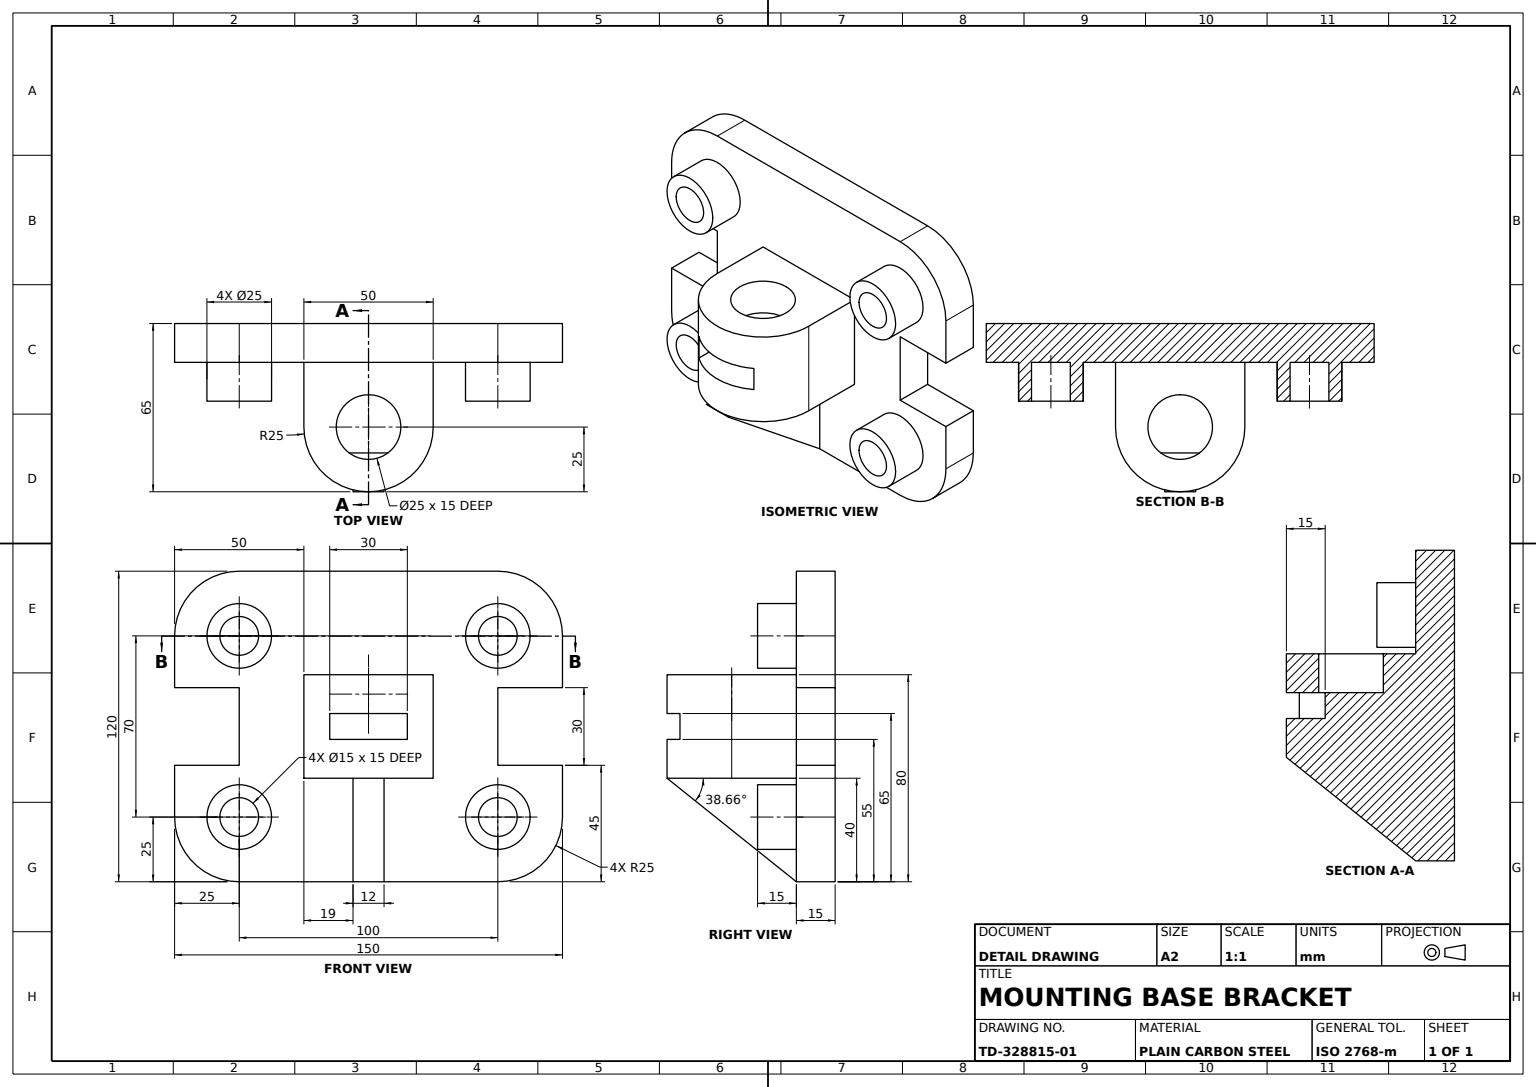
from build123d import *

# Parameters (mm, degrees)
BASE_PLATE_SKETCH_W         = 150
BASE_PLATE_SKETCH_H         = 120
BASE_PLATE_150X120X15_DEPTH = 15
RAISED_BOSS_SKETCH_R        = 12.5
RAISED_BOSS_SKETCH_R_2      = 7.5
RAISED_BOSS_15MM_DEPTH      = 15
BEARING_BLOCK_DEPTH         = 20
RELIEF_CUT_SKETCH_W         = 25
RELIEF_CUT_SKETCH_H         = 30
RELIEF_CUT_DEPTH            = 15
PLATE_CORNER_FILLETS_R25_R  = 25
BLOCK_SLOT_SKETCH_W         = 30
BLOCK_SLOT_SKETCH_H         = 10
BLOCK_SLOT_30X10_DEPTH      = 15
SUPPORT_RIB_DEPTH           = 6
BEARING_BORE_SKETCH_R       = 12.5
BEARING_BORE_25_DEPTH       = 15


with BuildPart() as part:
    # Base Plate Sketch → Base Plate 150x120x15 (new body)
    with BuildSketch(Plane.XY):
        with Locations((75, 60)):
            Rectangle(BASE_PLATE_SKETCH_W, BASE_PLATE_SKETCH_H)
    extrude(amount=BASE_PLATE_150X120X15_DEPTH)

    # Raised Boss Sketch → Raised Boss 15mm (add)
    # profile 1 of 4: a face of its own
    with BuildSketch(Plane.XY.offset(15)):
        with Locations((25, 95)):
            Circle(RAISED_BOSS_SKETCH_R)
        with Locations((25, 95)):
            Circle(RAISED_BOSS_SKETCH_R_2, mode=Mode.SUBTRACT)
    # profile 2 of 4: a face of its own
    with BuildSketch(Plane.XY.offset(15)):
        with Locations((125, 95)):
            Circle(RAISED_BOSS_SKETCH_R)
        with Locations((125, 95)):
            Circle(RAISED_BOSS_SKETCH_R_2, mode=Mode.SUBTRACT)
    # profile 3 of 4: a face of its own
    with BuildSketch(Plane.XY.offset(15)):
        with Locations((125, 25)):
            Circle(RAISED_BOSS_SKETCH_R)
        with Locations((125, 25)):
            Circle(RAISED_BOSS_SKETCH_R_2, mode=Mode.SUBTRACT)
    # profile 4 of 4: a face of its own
    with BuildSketch(Plane.XY.offset(15)):
        with Locations((25, 25)):
            Circle(RAISED_BOSS_SKETCH_R)
        with Locations((25, 25)):
            Circle(RAISED_BOSS_SKETCH_R_2, mode=Mode.SUBTRACT)
    extrude(amount=RAISED_BOSS_15MM_DEPTH)

    # Bearing Block Sketch → Bearing Block (add, symmetric)
    with BuildSketch(Plane(origin=(0, 60, 0), x_dir=(1, 0, 0), z_dir=(0, 1, 0))):
        with BuildLine():
            Line((50, -40), (50, -15))
            Line((50, -15), (100, -15))
            Line((100, -15), (100, -40))
            ThreePointArc((100, -40), (75, -65), (50, -40))
        make_face()
    extrude(amount=BEARING_BLOCK_DEPTH, both=True)

    # Relief Cut Sketch → Relief Cut (cut)
    with BuildSketch(Plane.XY.offset(15)):
        Polygon((150, 60), (150, 75), (125, 75), (125, 45), (150, 45), align=None)
        with Locations((12.5, 60)):
            Rectangle(RELIEF_CUT_SKETCH_W, RELIEF_CUT_SKETCH_H)
    extrude(amount=-RELIEF_CUT_DEPTH, mode=Mode.SUBTRACT)

    # Plate Corner Fillets R25
    plate_corner_fillets_r25_edges = [part.edges().sort_by_distance(p)[0] for p in [
        (0, 120, 7.5),
        (150, 120, 7.5),
        (150, 0, 7.5),
        (0, 0, 7.5),
    ]]
    fillet(plate_corner_fillets_r25_edges, radius=PLATE_CORNER_FILLETS_R25_R)

    # Block Slot Sketch → Block Slot 30x10 (cut)
    with BuildSketch(Plane.XY.offset(65)):
        with Locations((75, 60)):
            Rectangle(BLOCK_SLOT_SKETCH_W, BLOCK_SLOT_SKETCH_H)
    extrude(amount=-BLOCK_SLOT_30X10_DEPTH, mode=Mode.SUBTRACT)

    # Support Rib Sketch → Support Rib (add, symmetric)
    with BuildSketch(Plane(origin=(75, 0, 0), x_dir=(0, 0, -1), z_dir=(1, 0, 0))):
        Polygon((-15, 0), (-65, 40), (-15, 40), align=None)
    extrude(amount=SUPPORT_RIB_DEPTH, both=True)

    # Bearing Bore Sketch → Bearing Bore Ø25 (cut)
    with BuildSketch(Plane(origin=(0, 80, 0), x_dir=(1, 0, 0), z_dir=(0, 1, 0))):
        with Locations(Location((75, -40, 0), (0, 0, 270))):
            Circle(BEARING_BORE_SKETCH_R)
    extrude(amount=-BEARING_BORE_25_DEPTH, mode=Mode.SUBTRACT)


solid = part.part
